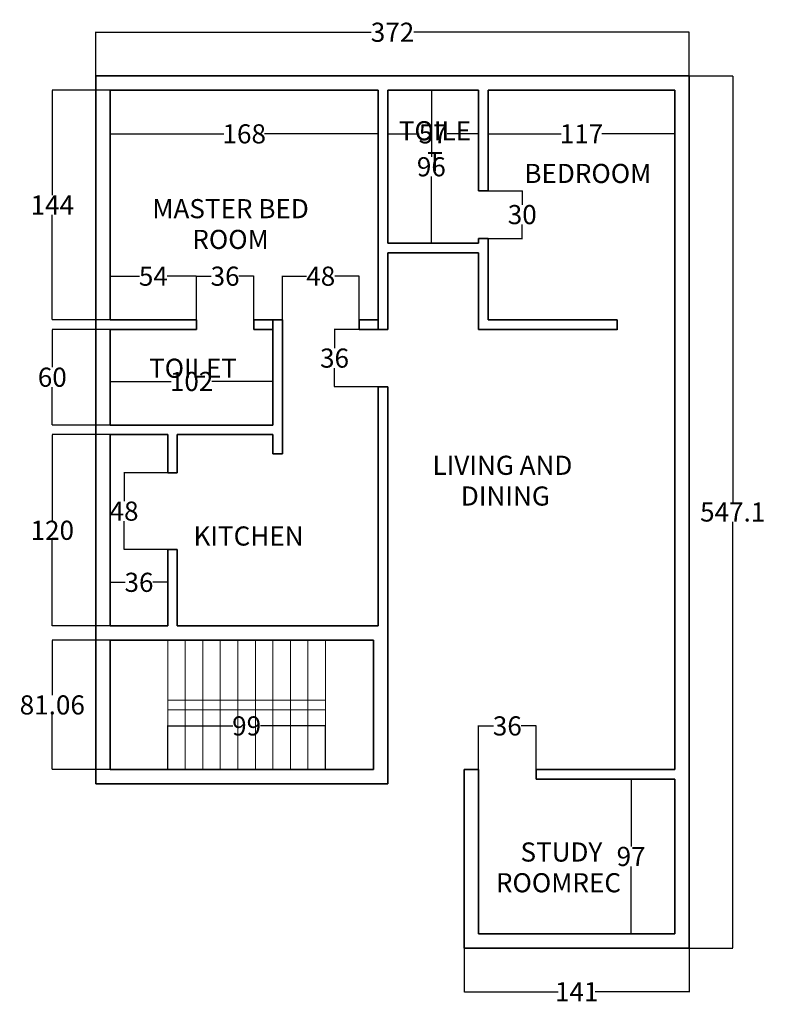
# Model space of a CAD drawing. Units: inches. Extents: x -24 to 1692, y -109 to 592.
# Tile 2 of 4: x 431 to 898, y -109 to 509. Entities that reach past the tile are written whole.
import ezdxf
from ezdxf.enums import TextEntityAlignment as Align

# ---------------------------------------------------------------- set-up
doc = ezdxf.new("R2010")
doc.units = ezdxf.units.IN
doc.header["$MEASUREMENT"] = 0
for name, color, linetype, lineweight in [('A-ANNO-DIMS', 2, 'Continuous', 18), ('A-AREA-IDEN', 7, 'Continuous', 18), ('A-FLOR-STRS', 2, 'Continuous', 18), ('A-WALL', 7, 'Continuous', 35)]:
    doc.layers.add(name, color=color, linetype=linetype, lineweight=lineweight)
doc.styles.get("Standard").update_dxf_attribs({"font": 'arial.ttf'})
doc.dimstyles.get("Standard").update_dxf_attribs({"dimtxt": 12, "dimasz": 0.18, "dimexe": 0.18, "dimexo": 0.0625, "dimgap": 0.09, "dimtad": 0, "dimtih": 1, "dimtoh": 1, "dimdec": 0, "dimzin": 0, "dimdsep": 46, "dimlunit": 4, "dimtxsty": 'Standard', "dimcen": 0.09, "dimadec": 0, "dimazin": 0, "dimtfac": 1, "dimtdec": 0, "dimtofl": 0, "dimtmove": 0, "dimatfit": 3, "dimfxl": 1, "dimtolj": 1, "dimtzin": 0, "dimarcsym": 0})

# ---------------------------------------------------------------- blocks, each defined once
blk = doc.blocks.new('*D33')
at = {"layer": 'A-ANNO-DIMS', "color": 0, "lineweight": -2, "transparency": 16777216}
for p, q in [((478.61, 473.42), (478.61, 500.91)), ((478.79, 500.73), (651.32, 500.73)), ((850.43, 500.73), (677.89, 500.73)), ((850.61, 473.42), (850.61, 500.91))]:
    blk.add_line(p, q, dxfattribs=at)
at = {"layer": 'A-ANNO-DIMS', "color": 0, "transparency": 16777216}
for points in [[(478.79, 500.76), (478.79, 500.7), (478.61, 500.73)], [(850.43, 500.76), (850.43, 500.7), (850.61, 500.73)]]:
    blk.add_solid(points, dxfattribs=at)
at = {"layer": 'Defpoints', "color": 0, "transparency": 16777216}
for p in [(850.61, 500.73), (478.61, 473.36), (850.61, 473.36)]:
    blk.add_point(p, dxfattribs=at)
at = {"layer": 'A-ANNO-DIMS', "color": 0, "transparency": 16777216, "insert": (664.61, 500.73), "char_height": 12, "attachment_point": 5}
blk.add_mtext('\\A1;372', dxfattribs=at)
blk = doc.blocks.new('*D34')
at = {"layer": 'A-ANNO-DIMS', "color": 0, "lineweight": -2, "transparency": 16777216}
for p, q in [((850.67, 473.36), (878.15, 473.36)), ((877.97, 473.18), (877.97, 206.05)), ((877.97, -73.52), (877.97, 193.61)), ((850.67, -73.7), (878.15, -73.7))]:
    blk.add_line(p, q, dxfattribs=at)
at = {"layer": 'A-ANNO-DIMS', "color": 0, "transparency": 16777216}
for points in [[(877.94, 473.18), (878, 473.18), (877.97, 473.36)], [(877.94, -73.52), (878, -73.52), (877.97, -73.7)]]:
    blk.add_solid(points, dxfattribs=at)
at = {"layer": 'Defpoints', "color": 0, "transparency": 16777216}
for p in [(850.61, 473.36), (877.97, 473.36), (850.61, -73.7)]:
    blk.add_point(p, dxfattribs=at)
at = {"layer": 'A-ANNO-DIMS', "color": 0, "transparency": 16777216, "insert": (877.97, 199.83), "char_height": 12, "attachment_point": 5}
blk.add_mtext('\\A1;547.1', dxfattribs=at)
blk = doc.blocks.new('*D35')
at = {"layer": 'A-ANNO-DIMS', "color": 0, "lineweight": -2, "transparency": 16777216}
for p, q in [((487.61, 464.3), (487.61, 436.82)), ((655.61, 464.3), (655.61, 436.82)), ((487.79, 437), (558.81, 437)), ((655.43, 437), (584.4, 437))]:
    blk.add_line(p, q, dxfattribs=at)
at = {"layer": 'A-ANNO-DIMS', "color": 0, "transparency": 16777216}
for points in [[(487.79, 437.03), (487.79, 436.97), (487.61, 437)], [(655.43, 437.03), (655.43, 436.97), (655.61, 437)]]:
    blk.add_solid(points, dxfattribs=at)
at = {"layer": 'Defpoints', "color": 0, "transparency": 16777216}
for p in [(487.61, 464.36), (655.61, 464.36), (487.61, 437)]:
    blk.add_point(p, dxfattribs=at)
at = {"layer": 'A-ANNO-DIMS', "color": 0, "transparency": 16777216, "insert": (571.61, 437), "char_height": 12, "attachment_point": 5}
blk.add_mtext('\\A1;168', dxfattribs=at)
blk = doc.blocks.new('*D36')
at = {"layer": 'A-ANNO-DIMS', "color": 0, "lineweight": -2, "transparency": 16777216}
for p, q in [((661.61, 464.3), (661.61, 436.82)), ((718.61, 464.3), (718.61, 436.82)), ((661.79, 437), (681.42, 437)), ((718.43, 437), (698.79, 437))]:
    blk.add_line(p, q, dxfattribs=at)
at = {"layer": 'A-ANNO-DIMS', "color": 0, "transparency": 16777216}
for points in [[(661.79, 437.03), (661.79, 436.97), (661.61, 437)], [(718.43, 437.03), (718.43, 436.97), (718.61, 437)]]:
    blk.add_solid(points, dxfattribs=at)
at = {"layer": 'Defpoints', "color": 0, "transparency": 16777216}
for p in [(661.61, 464.36), (718.61, 464.36), (661.61, 437)]:
    blk.add_point(p, dxfattribs=at)
at = {"layer": 'A-ANNO-DIMS', "color": 0, "transparency": 16777216, "insert": (690.11, 437), "char_height": 12, "attachment_point": 5}
blk.add_mtext('\\A1;57', dxfattribs=at)
blk = doc.blocks.new('*D37')
at = {"layer": 'A-ANNO-DIMS', "color": 0, "lineweight": -2, "transparency": 16777216}
for p, q in [((724.61, 464.3), (724.61, 436.82)), ((841.61, 464.3), (841.61, 436.82)), ((724.79, 437), (770.32, 437)), ((841.43, 437), (795.89, 437))]:
    blk.add_line(p, q, dxfattribs=at)
at = {"layer": 'A-ANNO-DIMS', "color": 0, "transparency": 16777216}
for points in [[(724.79, 437.03), (724.79, 436.97), (724.61, 437)], [(841.43, 437.03), (841.43, 436.97), (841.61, 437)]]:
    blk.add_solid(points, dxfattribs=at)
at = {"layer": 'Defpoints', "color": 0, "transparency": 16777216}
for p in [(724.61, 464.36), (841.61, 464.36), (724.61, 437)]:
    blk.add_point(p, dxfattribs=at)
at = {"layer": 'A-ANNO-DIMS', "color": 0, "transparency": 16777216, "insert": (783.11, 437), "char_height": 12, "attachment_point": 5}
blk.add_mtext('\\A1;117', dxfattribs=at)
blk = doc.blocks.new('*D38')
at = {"layer": 'A-ANNO-DIMS', "color": 0, "lineweight": -2, "transparency": 16777216}
for p, q in [((487.54, 464.36), (451.06, 464.36)), ((451.24, 464.18), (451.24, 398.48)), ((451.24, 320.54), (451.24, 386.25)), ((487.54, 320.36), (451.06, 320.36))]:
    blk.add_line(p, q, dxfattribs=at)
at = {"layer": 'A-ANNO-DIMS', "color": 0, "transparency": 16777216}
for points in [[(451.21, 464.18), (451.27, 464.18), (451.24, 464.36)], [(451.21, 320.54), (451.27, 320.54), (451.24, 320.36)]]:
    blk.add_solid(points, dxfattribs=at)
at = {"layer": 'Defpoints', "color": 0, "transparency": 16777216}
for p in [(451.24, 464.36), (487.61, 464.36), (487.61, 320.36)]:
    blk.add_point(p, dxfattribs=at)
at = {"layer": 'A-ANNO-DIMS', "color": 0, "transparency": 16777216, "insert": (451.24, 392.36), "char_height": 12, "attachment_point": 5}
blk.add_mtext('\\A1;144', dxfattribs=at)
blk = doc.blocks.new('*D39')
at = {"layer": 'A-ANNO-DIMS', "color": 0, "lineweight": -2, "transparency": 16777216}
for p, q in [((487.54, 314.36), (451.06, 314.36)), ((451.24, 314.18), (451.24, 290.58)), ((451.24, 254.54), (451.24, 278.15)), ((487.54, 254.36), (451.06, 254.36))]:
    blk.add_line(p, q, dxfattribs=at)
at = {"layer": 'A-ANNO-DIMS', "color": 0, "transparency": 16777216}
for points in [[(451.21, 314.18), (451.27, 314.18), (451.24, 314.36)], [(451.21, 254.54), (451.27, 254.54), (451.24, 254.36)]]:
    blk.add_solid(points, dxfattribs=at)
at = {"layer": 'Defpoints', "color": 0, "transparency": 16777216}
for p in [(451.24, 314.36), (487.61, 314.36), (487.61, 254.36)]:
    blk.add_point(p, dxfattribs=at)
at = {"layer": 'A-ANNO-DIMS', "color": 0, "transparency": 16777216, "insert": (451.24, 284.36), "char_height": 12, "attachment_point": 5}
blk.add_mtext('\\A1;60', dxfattribs=at)
blk = doc.blocks.new('*D40')
at = {"layer": 'A-ANNO-DIMS', "color": 0, "lineweight": -2, "transparency": 16777216}
for p, q in [((487.54, 248.36), (451.06, 248.36)), ((451.24, 248.18), (451.24, 194.58)), ((451.24, 128.54), (451.24, 182.15)), ((487.54, 128.36), (451.06, 128.36))]:
    blk.add_line(p, q, dxfattribs=at)
at = {"layer": 'A-ANNO-DIMS', "color": 0, "transparency": 16777216}
for points in [[(451.21, 248.18), (451.27, 248.18), (451.24, 248.36)], [(451.21, 128.54), (451.27, 128.54), (451.24, 128.36)]]:
    blk.add_solid(points, dxfattribs=at)
at = {"layer": 'Defpoints', "color": 0, "transparency": 16777216}
for p in [(451.24, 248.36), (487.61, 248.36), (487.61, 128.36)]:
    blk.add_point(p, dxfattribs=at)
at = {"layer": 'A-ANNO-DIMS', "color": 0, "transparency": 16777216, "insert": (451.24, 188.36), "char_height": 12, "attachment_point": 5}
blk.add_mtext('\\A1;120', dxfattribs=at)
blk = doc.blocks.new('*D41')
at = {"layer": 'A-ANNO-DIMS', "color": 0, "lineweight": -2, "transparency": 16777216}
for p, q in [((487.54, 119.36), (451.06, 119.36)), ((451.24, 119.18), (451.24, 85.05)), ((451.24, 38.48), (451.24, 72.61)), ((487.54, 38.3), (451.06, 38.3))]:
    blk.add_line(p, q, dxfattribs=at)
at = {"layer": 'A-ANNO-DIMS', "color": 0, "transparency": 16777216}
for points in [[(451.21, 119.18), (451.27, 119.18), (451.24, 119.36)], [(451.21, 38.48), (451.27, 38.48), (451.24, 38.3)]]:
    blk.add_solid(points, dxfattribs=at)
at = {"layer": 'Defpoints', "color": 0, "transparency": 16777216}
for p in [(451.24, 119.36), (487.61, 119.36), (487.61, 38.3)]:
    blk.add_point(p, dxfattribs=at)
at = {"layer": 'A-ANNO-DIMS', "color": 0, "transparency": 16777216, "insert": (451.24, 78.83), "char_height": 12, "attachment_point": 5}
blk.add_mtext('\\A1;81.06', dxfattribs=at)
blk = doc.blocks.new('*D42')
at = {"layer": 'A-ANNO-DIMS', "color": 0, "lineweight": -2, "transparency": 16777216}
for p, q in [((487.61, 254.42), (487.61, 281.91)), ((487.79, 281.73), (525.89, 281.73)), ((589.43, 281.73), (551.33, 281.73)), ((589.61, 254.42), (589.61, 281.91))]:
    blk.add_line(p, q, dxfattribs=at)
at = {"layer": 'A-ANNO-DIMS', "color": 0, "transparency": 16777216}
for points in [[(487.79, 281.76), (487.79, 281.7), (487.61, 281.73)], [(589.43, 281.76), (589.43, 281.7), (589.61, 281.73)]]:
    blk.add_solid(points, dxfattribs=at)
at = {"layer": 'Defpoints', "color": 0, "transparency": 16777216}
for p in [(589.61, 281.73), (487.61, 254.36), (589.61, 254.36)]:
    blk.add_point(p, dxfattribs=at)
at = {"layer": 'A-ANNO-DIMS', "color": 0, "transparency": 16777216, "insert": (538.61, 281.73), "char_height": 12, "attachment_point": 5}
blk.add_mtext('\\A1;102', dxfattribs=at)
blk = doc.blocks.new('*D43')
at = {"layer": 'A-ANNO-DIMS', "color": 0, "lineweight": -2, "transparency": 16777216}
for p, q in [((487.61, 128.42), (487.61, 155.91)), ((487.79, 155.73), (496.93, 155.73)), ((523.43, 155.73), (514.28, 155.73)), ((523.61, 128.42), (523.61, 155.91))]:
    blk.add_line(p, q, dxfattribs=at)
at = {"layer": 'A-ANNO-DIMS', "color": 0, "transparency": 16777216}
for points in [[(487.79, 155.76), (487.79, 155.7), (487.61, 155.73)], [(523.43, 155.76), (523.43, 155.7), (523.61, 155.73)]]:
    blk.add_solid(points, dxfattribs=at)
at = {"layer": 'Defpoints', "color": 0, "transparency": 16777216}
for p in [(523.61, 155.73), (487.61, 128.36), (523.61, 128.36)]:
    blk.add_point(p, dxfattribs=at)
at = {"layer": 'A-ANNO-DIMS', "color": 0, "transparency": 16777216, "insert": (505.61, 155.73), "char_height": 12, "attachment_point": 5}
blk.add_mtext('\\A1;36', dxfattribs=at)
blk = doc.blocks.new('*D44')
at = {"layer": 'A-ANNO-DIMS', "color": 0, "lineweight": -2, "transparency": 16777216}
for p, q in [((709.61, -73.76), (709.61, -101.25)), ((850.61, -73.76), (850.61, -101.25)), ((709.79, -101.07), (768.48, -101.07)), ((850.43, -101.07), (791.73, -101.07))]:
    blk.add_line(p, q, dxfattribs=at)
at = {"layer": 'A-ANNO-DIMS', "color": 0, "transparency": 16777216}
for points in [[(709.79, -101.04), (709.79, -101.1), (709.61, -101.07)], [(850.43, -101.04), (850.43, -101.1), (850.61, -101.07)]]:
    blk.add_solid(points, dxfattribs=at)
at = {"layer": 'Defpoints', "color": 0, "transparency": 16777216}
for p in [(709.61, -73.7), (850.61, -73.7), (850.61, -101.07)]:
    blk.add_point(p, dxfattribs=at)
at = {"layer": 'A-ANNO-DIMS', "color": 0, "transparency": 16777216, "insert": (780.11, -101.07), "char_height": 12, "attachment_point": 5}
blk.add_mtext('\\A1;141', dxfattribs=at)
blk = doc.blocks.new('*D45')
at = {"layer": 'A-ANNO-DIMS', "color": 0, "lineweight": -2, "transparency": 16777216}
for p, q in [((841.54, 32.3), (814.06, 32.3)), ((814.24, 32.12), (814.24, -9.98)), ((814.24, -64.52), (814.24, -22.42)), ((841.54, -64.7), (814.06, -64.7))]:
    blk.add_line(p, q, dxfattribs=at)
at = {"layer": 'A-ANNO-DIMS', "color": 0, "transparency": 16777216}
for points in [[(814.21, 32.12), (814.27, 32.12), (814.24, 32.3)], [(814.21, -64.52), (814.27, -64.52), (814.24, -64.7)]]:
    blk.add_solid(points, dxfattribs=at)
at = {"layer": 'Defpoints', "color": 0, "transparency": 16777216}
for p in [(814.24, 32.3), (841.61, 32.3), (841.61, -64.7)]:
    blk.add_point(p, dxfattribs=at)
at = {"layer": 'A-ANNO-DIMS', "color": 0, "transparency": 16777216, "insert": (814.24, -16.2), "char_height": 12, "attachment_point": 5}
blk.add_mtext('\\A1;97', dxfattribs=at)
blk = doc.blocks.new('*D46')
at = {"layer": 'A-ANNO-DIMS', "color": 0, "lineweight": -2, "transparency": 16777216}
for p, q in [((661.67, 464.36), (689.15, 464.36)), ((688.97, 464.18), (688.97, 422.58)), ((688.97, 368.54), (688.97, 410.15)), ((661.67, 368.36), (689.15, 368.36))]:
    blk.add_line(p, q, dxfattribs=at)
at = {"layer": 'A-ANNO-DIMS', "color": 0, "transparency": 16777216}
for points in [[(688.94, 464.18), (689, 464.18), (688.97, 464.36)], [(688.94, 368.54), (689, 368.54), (688.97, 368.36)]]:
    blk.add_solid(points, dxfattribs=at)
at = {"layer": 'Defpoints', "color": 0, "transparency": 16777216}
for p in [(661.61, 464.36), (661.61, 368.36), (688.97, 368.36)]:
    blk.add_point(p, dxfattribs=at)
at = {"layer": 'A-ANNO-DIMS', "color": 0, "transparency": 16777216, "insert": (688.97, 416.36), "char_height": 12, "attachment_point": 5}
blk.add_mtext('\\A1;96', dxfattribs=at)
blk = doc.blocks.new('*D47')
at = {"layer": 'A-ANNO-DIMS', "color": 0, "lineweight": -2, "transparency": 16777216}
for p, q in [((487.61, 320.42), (487.61, 347.91)), ((487.79, 347.73), (505.95, 347.73)), ((541.43, 347.73), (523.27, 347.73)), ((541.61, 320.42), (541.61, 347.91))]:
    blk.add_line(p, q, dxfattribs=at)
at = {"layer": 'A-ANNO-DIMS', "color": 0, "transparency": 16777216}
for points in [[(487.79, 347.76), (487.79, 347.7), (487.61, 347.73)], [(541.43, 347.76), (541.43, 347.7), (541.61, 347.73)]]:
    blk.add_solid(points, dxfattribs=at)
at = {"layer": 'Defpoints', "color": 0, "transparency": 16777216}
for p in [(541.61, 347.73), (487.61, 320.36), (541.61, 320.36)]:
    blk.add_point(p, dxfattribs=at)
at = {"layer": 'A-ANNO-DIMS', "color": 0, "transparency": 16777216, "insert": (514.61, 347.73), "char_height": 12, "attachment_point": 5}
blk.add_mtext('\\A1;54', dxfattribs=at)
blk = doc.blocks.new('*D48')
at = {"layer": 'A-ANNO-DIMS', "color": 0, "lineweight": -2, "transparency": 16777216}
for p, q in [((541.61, 320.42), (541.61, 347.91)), ((541.79, 347.73), (550.93, 347.73)), ((577.43, 347.73), (568.28, 347.73)), ((577.61, 320.42), (577.61, 347.91))]:
    blk.add_line(p, q, dxfattribs=at)
at = {"layer": 'A-ANNO-DIMS', "color": 0, "transparency": 16777216}
for points in [[(541.79, 347.76), (541.79, 347.7), (541.61, 347.73)], [(577.43, 347.76), (577.43, 347.7), (577.61, 347.73)]]:
    blk.add_solid(points, dxfattribs=at)
at = {"layer": 'Defpoints', "color": 0, "transparency": 16777216}
for p in [(577.61, 347.73), (541.61, 320.36), (577.61, 320.36)]:
    blk.add_point(p, dxfattribs=at)
at = {"layer": 'A-ANNO-DIMS', "color": 0, "transparency": 16777216, "insert": (559.61, 347.73), "char_height": 12, "attachment_point": 5}
blk.add_mtext('\\A1;36', dxfattribs=at)
blk = doc.blocks.new('*D49')
at = {"layer": 'A-ANNO-DIMS', "color": 0, "lineweight": -2, "transparency": 16777216}
for p, q in [((595.61, 320.42), (595.61, 347.91)), ((595.79, 347.73), (610.67, 347.73)), ((643.43, 347.73), (628.54, 347.73)), ((643.61, 320.42), (643.61, 347.91))]:
    blk.add_line(p, q, dxfattribs=at)
at = {"layer": 'A-ANNO-DIMS', "color": 0, "transparency": 16777216}
for points in [[(595.79, 347.76), (595.79, 347.7), (595.61, 347.73)], [(643.43, 347.76), (643.43, 347.7), (643.61, 347.73)]]:
    blk.add_solid(points, dxfattribs=at)
at = {"layer": 'Defpoints', "color": 0, "transparency": 16777216}
for p in [(643.61, 347.73), (595.61, 320.36), (643.61, 320.36)]:
    blk.add_point(p, dxfattribs=at)
at = {"layer": 'A-ANNO-DIMS', "color": 0, "transparency": 16777216, "insert": (619.61, 347.73), "char_height": 12, "attachment_point": 5}
blk.add_mtext('\\A1;48', dxfattribs=at)
blk = doc.blocks.new('*D50')
at = {"layer": 'A-ANNO-DIMS', "color": 0, "lineweight": -2, "transparency": 16777216}
for p, q in [((718.67, 401.36), (746.15, 401.36)), ((745.97, 401.18), (745.97, 392.58)), ((745.97, 371.54), (745.97, 380.14)), ((718.67, 371.36), (746.15, 371.36))]:
    blk.add_line(p, q, dxfattribs=at)
at = {"layer": 'A-ANNO-DIMS', "color": 0, "transparency": 16777216}
for points in [[(745.94, 401.18), (746, 401.18), (745.97, 401.36)], [(745.94, 371.54), (746, 371.54), (745.97, 371.36)]]:
    blk.add_solid(points, dxfattribs=at)
at = {"layer": 'Defpoints', "color": 0, "transparency": 16777216}
for p in [(718.61, 401.36), (718.61, 371.36), (745.97, 371.36)]:
    blk.add_point(p, dxfattribs=at)
at = {"layer": 'A-ANNO-DIMS', "color": 0, "transparency": 16777216, "insert": (745.97, 386.36), "char_height": 12, "attachment_point": 5}
blk.add_mtext('\\A1;30', dxfattribs=at)
blk = doc.blocks.new('*D51')
at = {"layer": 'A-ANNO-DIMS', "color": 0, "lineweight": -2, "transparency": 16777216}
for p, q in [((655.54, 314.36), (628.06, 314.36)), ((628.24, 314.18), (628.24, 302.58)), ((628.24, 278.54), (628.24, 290.14)), ((655.54, 278.36), (628.06, 278.36))]:
    blk.add_line(p, q, dxfattribs=at)
at = {"layer": 'A-ANNO-DIMS', "color": 0, "transparency": 16777216}
for points in [[(628.21, 314.18), (628.27, 314.18), (628.24, 314.36)], [(628.21, 278.54), (628.27, 278.54), (628.24, 278.36)]]:
    blk.add_solid(points, dxfattribs=at)
at = {"layer": 'Defpoints', "color": 0, "transparency": 16777216}
for p in [(628.24, 314.36), (655.61, 314.36), (655.61, 278.36)]:
    blk.add_point(p, dxfattribs=at)
at = {"layer": 'A-ANNO-DIMS', "color": 0, "transparency": 16777216, "insert": (628.24, 296.36), "char_height": 12, "attachment_point": 5}
blk.add_mtext('\\A1;36', dxfattribs=at)
blk = doc.blocks.new('*D52')
at = {"layer": 'A-ANNO-DIMS', "color": 0, "lineweight": -2, "transparency": 16777216}
for p, q in [((523.54, 224.36), (496.06, 224.36)), ((496.24, 224.18), (496.24, 206.58)), ((496.24, 176.54), (496.24, 194.15)), ((523.54, 176.36), (496.06, 176.36))]:
    blk.add_line(p, q, dxfattribs=at)
at = {"layer": 'A-ANNO-DIMS', "color": 0, "transparency": 16777216}
for points in [[(496.21, 224.18), (496.27, 224.18), (496.24, 224.36)], [(496.21, 176.54), (496.27, 176.54), (496.24, 176.36)]]:
    blk.add_solid(points, dxfattribs=at)
at = {"layer": 'Defpoints', "color": 0, "transparency": 16777216}
for p in [(496.24, 224.36), (523.61, 224.36), (523.61, 176.36)]:
    blk.add_point(p, dxfattribs=at)
at = {"layer": 'A-ANNO-DIMS', "color": 0, "transparency": 16777216, "insert": (496.24, 200.36), "char_height": 12, "attachment_point": 5}
blk.add_mtext('\\A1;48', dxfattribs=at)
blk = doc.blocks.new('*D53')
at = {"layer": 'A-ANNO-DIMS', "color": 0, "lineweight": -2, "transparency": 16777216}
for p, q in [((523.61, 38.36), (523.61, 65.84)), ((523.79, 65.66), (564.41, 65.66)), ((622.43, 65.66), (581.8, 65.66)), ((622.61, 38.36), (622.61, 65.84))]:
    blk.add_line(p, q, dxfattribs=at)
at = {"layer": 'A-ANNO-DIMS', "color": 0, "transparency": 16777216}
for points in [[(523.79, 65.69), (523.79, 65.63), (523.61, 65.66)], [(622.43, 65.69), (622.43, 65.63), (622.61, 65.66)]]:
    blk.add_solid(points, dxfattribs=at)
at = {"layer": 'Defpoints', "color": 0, "transparency": 16777216}
for p in [(622.61, 65.66), (523.61, 38.3), (622.61, 38.3)]:
    blk.add_point(p, dxfattribs=at)
at = {"layer": 'A-ANNO-DIMS', "color": 0, "transparency": 16777216, "insert": (573.11, 65.66), "char_height": 12, "attachment_point": 5}
blk.add_mtext('\\A1;99', dxfattribs=at)
blk = doc.blocks.new('*D54')
at = {"layer": 'A-ANNO-DIMS', "color": 0, "lineweight": -2, "transparency": 16777216}
for p, q in [((718.61, 38.36), (718.61, 65.84)), ((718.79, 65.66), (727.93, 65.66)), ((754.43, 65.66), (745.28, 65.66)), ((754.61, 38.36), (754.61, 65.84))]:
    blk.add_line(p, q, dxfattribs=at)
at = {"layer": 'A-ANNO-DIMS', "color": 0, "transparency": 16777216}
for points in [[(718.79, 65.69), (718.79, 65.63), (718.61, 65.66)], [(754.43, 65.69), (754.43, 65.63), (754.61, 65.66)]]:
    blk.add_solid(points, dxfattribs=at)
at = {"layer": 'Defpoints', "color": 0, "transparency": 16777216}
for p in [(754.61, 65.66), (718.61, 38.3), (754.61, 38.3)]:
    blk.add_point(p, dxfattribs=at)
at = {"layer": 'A-ANNO-DIMS', "color": 0, "transparency": 16777216, "insert": (736.61, 65.66), "char_height": 12, "attachment_point": 5}
blk.add_mtext('\\A1;36', dxfattribs=at)

msp = doc.modelspace()

# ---------------------------------------------------------------- linework, layer by layer
at = {"layer": 'A-FLOR-STRS'}
for p, q in [((523.6054, 119.3621), (523.6054, 38.2996)), ((534.6054, 119.3621), (534.6054, 38.2996)), ((545.6054, 119.3621), (545.6054, 38.2996)), ((556.6054, 119.3621), (556.6054, 38.2996)), ((567.6054, 119.3621), (567.6054, 38.2996)), ((578.6054, 119.3621), (578.6054, 38.2996)), ((589.6054, 119.3621), (589.6054, 38.2996)), ((600.6054, 119.3621), (600.6054, 38.2996)), ((611.6054, 119.3621), (611.6054, 38.2996)), ((622.6054, 119.3621), (622.6054, 38.2996)), ((622.6054, 81.8621), (523.6054, 81.8621)), ((523.6054, 75.7996), (622.6054, 75.7996))]:
    msp.add_line(p, q, dxfattribs=at)
at = {"layer": 'A-WALL'}
for p, q in [((850.6054, 473.3621), (478.6054, 473.3621)), ((478.6054, 473.3621), (478.6054, 29.2996)), ((850.6054, -73.7004), (850.6054, 473.3621)), ((487.6054, 464.3621), (487.6054, 320.3621)), ((655.6054, 464.3621), (487.6054, 464.3621)), ((655.6054, 464.3621), (655.6054, 320.3621)), ((661.6054, 464.3621), (661.6054, 368.3621)), ((718.6054, 464.3621), (661.6054, 464.3621)), ((718.6054, 464.3621), (718.6054, 401.3621)), ((841.6054, 464.3621), (724.6054, 464.3621)), ((724.6054, 464.3621), (724.6054, 401.3621)), ((841.6054, 320.3621), (841.6054, 464.3621)), ((718.6054, 401.3621), (724.6054, 401.3621)), ((718.6054, 371.3621), (724.6054, 371.3621)), ((718.6054, 371.3621), (718.6054, 368.3621)), ((724.6054, 371.3621), (724.6054, 320.3621)), ((718.6054, 368.3621), (661.6054, 368.3621)), ((718.6054, 362.3621), (661.6054, 362.3621)), ((661.6054, 362.3621), (661.6054, 314.3621)), ((718.6054, 362.3621), (718.6054, 314.3621)), ((541.6054, 320.3621), (487.6054, 320.3621)), ((541.6054, 314.3621), (541.6054, 320.3621)), ((595.6054, 320.3621), (577.6054, 320.3621)), ((577.6054, 314.3621), (577.6054, 320.3621)), ((589.6054, 314.3621), (589.6054, 320.3621)), ((595.6054, 320.3621), (595.6054, 236.3621)), ((655.6054, 320.3621), (643.6054, 320.3621)), ((643.6054, 320.3621), (643.6054, 314.3621)), ((655.6054, 320.3621), (655.6054, 314.3621)), ((805.6054, 320.3621), (724.6054, 320.3621)), ((805.6054, 320.3621), (805.6054, 314.1117)), ((841.6054, 320.3621), (841.6054, 314.1117)), ((487.6054, 314.3621), (487.6054, 254.3621)), ((541.6054, 314.3621), (487.6054, 314.3621)), ((589.6054, 314.3621), (577.6054, 314.3621)), ((589.6054, 314.3621), (589.6054, 254.3621)), ((655.6054, 314.3621), (643.6054, 314.3621)), ((655.6054, 314.3621), (661.6054, 314.3621)), ((805.6054, 314.3621), (718.6054, 314.3621)), ((841.6054, 38.2996), (841.6054, 314.3621)), ((655.6054, 278.3621), (655.6054, 128.3621)), ((655.6054, 278.3621), (661.6054, 278.3621)), ((661.6054, 278.3621), (661.6054, 29.2996)), ((589.6054, 254.3621), (487.6054, 254.3621)), ((487.6054, 248.3621), (487.6054, 128.3621)), ((523.6054, 248.3621), (487.6054, 248.3621)), ((523.6054, 248.3621), (523.6054, 224.3621)), ((589.6054, 248.3621), (529.6054, 248.3621)), ((529.6054, 248.3621), (529.6054, 224.3621)), ((589.6054, 248.3621), (589.6054, 236.3621)), ((589.6054, 236.3621), (595.6054, 236.3621)), ((523.6054, 224.3621), (529.6054, 224.3621)), ((523.6054, 176.3621), (529.6054, 176.3621)), ((523.6054, 176.3621), (523.6054, 128.3621)), ((529.6054, 176.3621), (529.6054, 128.3621)), ((523.6054, 128.3621), (487.6054, 128.3621)), ((655.6054, 128.3621), (529.6054, 128.3621)), ((652.6054, 119.3621), (487.6054, 119.3621)), ((487.6054, 119.3621), (487.6054, 38.2996)), ((652.6054, 119.3621), (652.6054, 38.2996)), ((487.6054, 38.2996), (652.6054, 38.2996)), ((529.6054, 38.2996), (652.6054, 38.2996)), ((709.6054, 38.2996), (718.6054, 38.2996)), ((709.6054, 38.2996), (718.6054, 38.2996)), ((709.6054, 38.2996), (709.6054, -73.7004)), ((718.6054, 29.2996), (718.6054, 38.2996)), ((754.6054, 38.2996), (841.6054, 38.2996)), ((754.6054, 32.2996), (754.6054, 38.2996)), ((754.6054, 38.2996), (841.6054, 38.2996)), ((754.6054, 32.2996), (841.6054, 32.2996)), ((841.6054, -64.7004), (841.6054, 32.2996)), ((478.6054, 29.2996), (661.6054, 29.2996)), ((718.6054, 29.2996), (718.6054, -64.7004)), ((718.6054, -64.7004), (841.6054, -64.7004)), ((709.6054, -73.7004), (850.6054, -73.7004))]:
    msp.add_line(p, q, dxfattribs=at)

# ---------------------------------------------------------------- texts
at = {"layer": 'A-AREA-IDEN'}
for s, p in [('TOILE', (691.2042, 432.9374)), ('T', (691.2042, 413.6605)), ('BEDROOM', (787.1263, 406.1719)), ('MASTER BED', (563.0339, 384.0772)), ('ROOM', (563.0339, 364.8003)), ('TOILET', (539.4821, 283.9928)), ('LIVING AND', (733.5482, 223.1302)), (' DINING', (733.5482, 203.8533)), ('KITCHEN', (574.2959, 178.7736)), ('STUDY', (770.5287, -19.4175)), ('ROOMREC ', (770.5287, -38.6944))]:
    msp.add_text(s, height=12, dxfattribs=at).set_placement(p, align=Align.CENTER)

# ---------------------------------------------------------------- dimensions: what is measured, and where the dimension line sits
at = {"layer": 'A-ANNO-DIMS'}
for base, p1, p2, picture, middle in [((850.6054, 500.7271), (478.6054, 473.3621), (850.6054, 473.3621), '*D33', (664.6054, 500.7271)), ((541.6054, 347.7271), (487.6054, 320.3621), (541.6054, 320.3621), '*D47', (514.6054, 347.7271)), ((577.6054, 347.7271), (541.6054, 320.3621), (577.6054, 320.3621), '*D48', (559.6054, 347.7271)), ((643.6054, 347.7271), (595.6054, 320.3621), (643.6054, 320.3621), '*D49', (619.6054, 347.7271)), ((589.6054, 281.7271), (487.6054, 254.3621), (589.6054, 254.3621), '*D42', (538.6054, 281.7271)), ((523.6054, 155.7271), (487.6054, 128.3621), (523.6054, 128.3621), '*D43', (505.6054, 155.7271)), ((622.6054, 65.6646), (523.6054, 38.2996), (622.6054, 38.2996), '*D53', (573.1054, 65.6646)), ((754.6054, 65.6646), (718.6054, 38.2996), (754.6054, 38.2996), '*D54', (736.6054, 65.6646)), ((850.6054, -101.0654), (709.6054, -73.7004), (850.6054, -73.7004), '*D44', (780.1054, -101.0654))]:
    dim = msp.add_linear_dim(base=base, p1=p1, p2=p2, dimstyle='Standard', override={"dimdec": 0, "dimlfac": 1, "dimrnd": 0, "dimzin": 0, "dimdsep": 46, "dimlunit": 2}, dxfattribs=at)
    dim.commit()
    dim.dimension.update_dxf_attribs({"geometry": picture, "text_midpoint": middle})
for base, p1, p2, angle, override, picture, middle in [((877.9704, 473.3621), (850.6054, -73.7004), (850.6054, 473.3621), 90, {"dimdec": 1, "dimlfac": 1, "dimrnd": 0, "dimzin": 0, "dimdsep": 46, "dimlunit": 2}, '*D34', (877.9704, 199.8308)), ((451.2404, 464.3621), (487.6054, 320.3621), (487.6054, 464.3621), 90, {"dimdec": 0, "dimlfac": 1, "dimrnd": 0, "dimzin": 0, "dimdsep": 46, "dimlunit": 2}, '*D38', (451.2404, 392.3621)), ((487.6054, 436.9971), (655.6054, 464.3621), (487.6054, 464.3621), 180, {"dimdec": 0, "dimlfac": 1, "dimrnd": 0, "dimzin": 0, "dimdsep": 46, "dimlunit": 2}, '*D35', (571.6054, 436.9971)), ((661.6054, 436.9971), (718.6054, 464.3621), (661.6054, 464.3621), 180, {"dimdec": 0, "dimlfac": 1, "dimrnd": 0, "dimzin": 0, "dimdsep": 46, "dimlunit": 2}, '*D36', (690.1054, 436.9971)), ((688.9704, 368.3621), (661.6054, 464.3621), (661.6054, 368.3621), 270, {"dimdec": 0, "dimlfac": 1, "dimrnd": 0, "dimzin": 0, "dimdsep": 46, "dimlunit": 2}, '*D46', (688.9704, 416.3621)), ((724.6054, 436.9971), (841.6054, 464.3621), (724.6054, 464.3621), 180, {"dimdec": 0, "dimlfac": 1, "dimrnd": 0, "dimzin": 0, "dimdsep": 46, "dimlunit": 2}, '*D37', (783.1054, 436.9971)), ((745.9704, 371.3621), (718.6054, 401.3621), (718.6054, 371.3621), 270, {"dimdec": 0, "dimlfac": 1, "dimrnd": 0, "dimzin": 0, "dimdsep": 46, "dimlunit": 2}, '*D50', (745.9704, 386.3621)), ((451.2404, 314.3621), (487.6054, 254.3621), (487.6054, 314.3621), 90, {"dimdec": 0, "dimlfac": 1, "dimrnd": 0, "dimzin": 0, "dimdsep": 46, "dimlunit": 2}, '*D39', (451.2404, 284.3621)), ((628.2404, 314.3621), (655.6054, 278.3621), (655.6054, 314.3621), 90, {"dimdec": 0, "dimlfac": 1, "dimrnd": 0, "dimzin": 0, "dimdsep": 46, "dimlunit": 2}, '*D51', (628.2404, 296.3621)), ((451.2404, 248.3621), (487.6054, 128.3621), (487.6054, 248.3621), 90, {"dimdec": 0, "dimlfac": 1, "dimrnd": 0, "dimzin": 0, "dimdsep": 46, "dimlunit": 2}, '*D40', (451.2404, 188.3621)), ((496.2404, 224.3621), (523.6054, 176.3621), (523.6054, 224.3621), 90, {"dimdec": 0, "dimlfac": 1, "dimrnd": 0, "dimzin": 0, "dimdsep": 46, "dimlunit": 2}, '*D52', (496.2404, 200.3621)), ((451.2404, 119.3621), (487.6054, 38.2996), (487.6054, 119.3621), 90, {"dimdec": 2, "dimlfac": 1, "dimrnd": 0, "dimzin": 0, "dimdsep": 46, "dimlunit": 2}, '*D41', (451.2404, 78.8308)), ((814.2404, 32.2996), (841.6054, -64.7004), (841.6054, 32.2996), 90, {"dimdec": 0, "dimlfac": 1, "dimrnd": 0, "dimzin": 0, "dimdsep": 46, "dimlunit": 2}, '*D45', (814.2404, -16.2004))]:
    dim = msp.add_linear_dim(base=base, p1=p1, p2=p2, angle=angle, dimstyle='Standard', override=override, dxfattribs=at)
    dim.commit()
    dim.dimension.update_dxf_attribs({"geometry": picture, "text_midpoint": middle})

doc.saveas('drawing.dxf')
